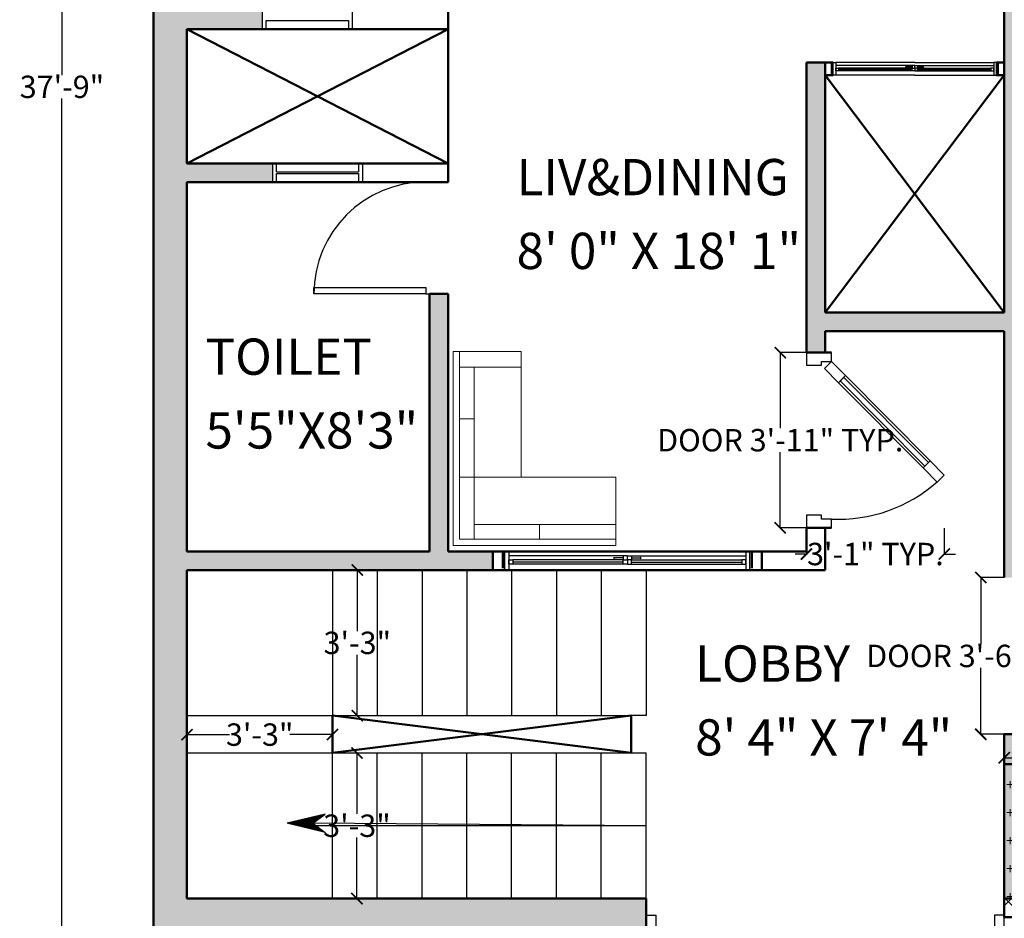
# Model space of a CAD drawing. Units: inches. Extents: x 2278 to 7495, y -71 to 1198.
# Tile 2 of 44: x 2278 to 2542, y 714 to 955. Entities that reach past the tile are written whole.
import ezdxf

# ---------------------------------------------------------------- set-up
doc = ezdxf.new("R2010")
doc.units = ezdxf.units.IN
doc.header["$MEASUREMENT"] = 0
for name, color, linetype, lineweight in [('A-ANNO-DIMS', 2, 'Continuous', 18), ('A-AREA-IDEN', 3, 'Continuous', 18), ('A-Door', 3, 'Continuous', 25), ('A-FLOR-PATT', 252, 'Continuous', 13), ('A-FLOR-STRS', 6, 'Continuous', 25), ('A-FURN', 8, 'Continuous', 18), ('A-Glaz', 4, 'Continuous', 25), ('A-Wall', 7, 'Continuous', 50), ('A-WALL-PATT', 8, 'Continuous', 18)]:
    doc.layers.add(name, color=color, linetype=linetype, lineweight=lineweight)
doc.styles.get("Standard").update_dxf_attribs({"font": 'arial.ttf'})
doc.dimstyles.get("Standard").update_dxf_attribs({"dimtxt": 6, "dimasz": 3, "dimexe": 0.18, "dimexo": 0.0625, "dimgap": 0.09, "dimtad": 0, "dimtih": 1, "dimtoh": 1, "dimdec": 0, "dimzin": 0, "dimdsep": 46, "dimlunit": 3, "dimtxsty": 'Standard', "dimblk": 'ARCHTICK', "dimcen": 0.09, "dimadec": 0, "dimazin": 0, "dimtfac": 1, "dimtdec": 0, "dimtofl": 0, "dimtmove": 0, "dimatfit": 3, "dimfxl": 1, "dimtolj": 1, "dimtzin": 0, "dimarcsym": 0})

# ---------------------------------------------------------------- blocks, each defined once
blk = doc.blocks.new('*U5')
for p, q in [((0, 0), (0, -6)), ((30, 0), (30, -6))]:
    blk.add_line(p, q)
blk.add_lwpolyline([(0, 0), (0, 30), (1.75, 30), (1.75, 0)], close=True)
blk.add_arc((0, 0), 30, 0, 90)
blk = doc.blocks.new('A$C58286AE3')
for p, q in [((75, 820), (35, 820)), ((35, 820), (35, 180)), ((65, 820), (45, 820)), ((75, 180), (75, 820)), ((75, 180), (35, 180)), ((35, 180), (75, 180)), ((45, 180), (65, 180))]:
    blk.add_line(p, q)
blk.add_lwpolyline([(1725, 180), (1725, 820), (1765, 820), (1765, 180)], close=True)
blk.add_arc((1756.5, 42.1), 858.5, 92.1038, 176.1334)
blk.add_ellipse((70, 105), major_axis=(-772.1, 325.5), ratio=0.94084, start_param=-2.726592, end_param=-1.199193)
at = {"layer": 'A-Door'}
for p, q in [((35, 820), (35, 900)), ((35, 900), (75, 900)), ((75, 900), (75, 820)), ((75, 820), (35, 820)), ((35, 180), (35, 100)), ((75, 100), (75, 180)), ((35, 100), (0, 100)), ((0, 100), (0, 0)), ((35, 60), (35, 100)), ((35, 100), (75, 100)), ((50, 60), (35, 60)), ((50, 50), (50, 60)), ((50, 0), (50, 50)), ((0, 0), (50, 0))]:
    blk.add_line(p, q, dxfattribs=at)
for points in [[(1725, 900), (1725, 820), (1765, 820), (1765, 900)], [(1725, 100), (1725, 180), (1765, 180), (1765, 100)], [(1765, 100), (1800, 100), (1800, 0), (1750, 0), (1750, 50), (1750, 60), (1765, 60)]]:
    blk.add_lwpolyline(points, close=True, dxfattribs=at)
at = {"layer": 'A-Glaz'}
for p, q in [((45, 820), (45, 180)), ((65, 180), (65, 820))]:
    blk.add_line(p, q, dxfattribs=at)
blk.add_lwpolyline([(1735, 180), (1735, 820), (1755, 820), (1755, 180)], close=True, dxfattribs=at)
blk = doc.blocks.new('A$C1DF4181C')
blk.add_lwpolyline([(120, 128), (460.7, 466.1), (432.5, 494.5), (91.8, 156.4)], close=True)
blk.add_arc((72.4, 128.7), 593.3, 357.2313, 41.4937)
at = {"layer": 'A-Door'}
for points in [[(517.5, 522.4), (460.7, 466.1), (432.5, 494.5), (489.3, 550.8)], [(63.2, 71.6), (120, 128), (91.8, 156.4), (35, 100)], [(35, 100), (0, 100), (0, 0), (50, 0), (50, 50), (50, 60), (35, 60)], [(665, 100), (665, 60), (650, 60), (650, 50), (650, 0), (700, 0), (700, 100)]]:
    blk.add_lwpolyline(points, close=True, dxfattribs=at)
at = {"layer": 'A-Glaz'}
blk.add_lwpolyline([(112.9, 135.1), (453.6, 473.2), (439.5, 487.4), (98.8, 149.3)], close=True, dxfattribs=at)
at = {"layer": 'A-Wall'}
for p, q in [((0, 0), (0, 100)), ((0, 100), (0, 0)), ((700, 0), (700, 100)), ((700, 0), (700, 100))]:
    blk.add_line(p, q, dxfattribs=at)
blk = doc.blocks.new('_ArchTick')
at = {"color": 0, "linetype": 'ByBlock', "const_width": 0.15}
blk.add_lwpolyline([(-0.5, -0.5), (0.5, 0.5)], dxfattribs=at)
blk = doc.blocks.new('*D11')
at = {"layer": 'A-ANNO-DIMS', "color": 0, "lineweight": -2, "transparency": 16777216}
for p, q in [((2367.65, 807.47), (2368.7, 807.47)), ((2368.52, 807.47), (2368.52, 791.12)), ((2368.52, 768.47), (2368.52, 784.81)), ((2367.65, 768.47), (2368.7, 768.47))]:
    blk.add_line(p, q, dxfattribs=at)
at = {"layer": 'Defpoints', "color": 0, "transparency": 16777216}
for p in [(2367.59, 807.47), (2367.59, 768.47), (2368.52, 768.47)]:
    blk.add_point(p, dxfattribs=at)
at = {"layer": 'A-ANNO-DIMS', "color": 0, "lineweight": -2, "transparency": 16777216, "xscale": 3, "yscale": 3, "zscale": 3}
for p, rotation in [((2368.52, 807.47), 90), ((2368.52, 768.47), 270)]:
    blk.add_blockref('_ArchTick', p, dxfattribs=dict(at, rotation=rotation))
at = {"layer": 'A-ANNO-DIMS', "color": 0, "transparency": 16777216, "insert": (2368.52, 787.97), "char_height": 6, "attachment_point": 5}
blk.add_mtext('\\A1;3\'-3"', dxfattribs=at)
blk = doc.blocks.new('*D12')
at = {"layer": 'A-ANNO-DIMS', "color": 0, "lineweight": -2, "transparency": 16777216}
for p, q in [((2322.87, 763.4), (2322.87, 763.21)), ((2322.87, 763.39), (2334.31, 763.39)), ((2361.87, 763.39), (2350.43, 763.39)), ((2361.87, 763.4), (2361.87, 763.21))]:
    blk.add_line(p, q, dxfattribs=at)
at = {"layer": 'Defpoints', "color": 0, "transparency": 16777216}
for p in [(2322.87, 763.47), (2361.87, 763.47), (2361.87, 763.39)]:
    blk.add_point(p, dxfattribs=at)
at = {"layer": 'A-ANNO-DIMS', "color": 0, "lineweight": -2, "transparency": 16777216, "xscale": 3, "yscale": 3, "zscale": 3, "rotation": 180}
blk.add_blockref('_ArchTick', (2322.87, 763.39), dxfattribs=at)
at = {"layer": 'A-ANNO-DIMS', "color": 0, "lineweight": -2, "transparency": 16777216, "xscale": 3, "yscale": 3, "zscale": 3}
blk.add_blockref('_ArchTick', (2361.87, 763.39), dxfattribs=at)
at = {"layer": 'A-ANNO-DIMS', "color": 0, "transparency": 16777216, "insert": (2342.37, 763.39), "char_height": 6, "attachment_point": 5}
blk.add_mtext('\\A1;3\'-3"', dxfattribs=at)
blk = doc.blocks.new('*D13')
at = {"layer": 'A-ANNO-DIMS', "color": 0, "lineweight": -2, "transparency": 16777216}
for p, q in [((2367.61, 758.47), (2368.61, 758.47)), ((2368.43, 758.47), (2368.43, 742.12)), ((2368.43, 719.47), (2368.43, 735.81)), ((2367.61, 719.47), (2368.61, 719.47))]:
    blk.add_line(p, q, dxfattribs=at)
at = {"layer": 'Defpoints', "color": 0, "transparency": 16777216}
for p in [(2367.55, 758.47), (2367.55, 719.47), (2368.43, 719.47)]:
    blk.add_point(p, dxfattribs=at)
at = {"layer": 'A-ANNO-DIMS', "color": 0, "lineweight": -2, "transparency": 16777216, "xscale": 3, "yscale": 3, "zscale": 3}
for p, rotation in [((2368.43, 758.47), 90), ((2368.43, 719.47), 270)]:
    blk.add_blockref('_ArchTick', p, dxfattribs=dict(at, rotation=rotation))
at = {"layer": 'A-ANNO-DIMS', "color": 0, "transparency": 16777216, "insert": (2368.43, 738.97), "char_height": 6, "attachment_point": 5}
blk.add_mtext('\\A1;3\'-3"', dxfattribs=at)
blk = doc.blocks.new('*D17')
at = {"layer": 'A-ANNO-DIMS', "color": 0, "lineweight": -2, "transparency": 16777216}
for p, q in [((2313.81, 1163.47), (2289.2, 1163.47)), ((2289.38, 1163.47), (2289.38, 940.12)), ((2289.38, 710.47), (2289.38, 933.81)), ((2313.81, 710.47), (2289.2, 710.47))]:
    blk.add_line(p, q, dxfattribs=at)
at = {"layer": 'Defpoints', "color": 0, "transparency": 16777216}
for p in [(2313.87, 1163.47), (2289.38, 710.47), (2313.87, 710.47)]:
    blk.add_point(p, dxfattribs=at)
at = {"layer": 'A-ANNO-DIMS', "color": 0, "lineweight": -2, "transparency": 16777216, "xscale": 3, "yscale": 3, "zscale": 3}
for p, rotation in [((2289.38, 1163.47), 90), ((2289.38, 710.47), 270)]:
    blk.add_blockref('_ArchTick', p, dxfattribs=dict(at, rotation=rotation))
at = {"layer": 'A-ANNO-DIMS', "color": 0, "transparency": 16777216, "insert": (2289.38, 936.97), "char_height": 6, "attachment_point": 5}
blk.add_mtext('\\A1;37\'-9"', dxfattribs=at)
blk = doc.blocks.new('*D43')
at = {"layer": 'A-ANNO-DIMS', "color": 0, "lineweight": -2, "transparency": 16777216}
for p, q in [((2541.81, 805.47), (2535.39, 805.47)), ((2535.57, 805.47), (2535.57, 787.66)), ((2535.57, 763.47), (2535.57, 781.27)), ((2541.81, 763.47), (2535.39, 763.47))]:
    blk.add_line(p, q, dxfattribs=at)
at = {"layer": 'Defpoints', "color": 0, "transparency": 16777216}
for p in [(2541.87, 805.47), (2535.57, 763.47), (2541.87, 763.47)]:
    blk.add_point(p, dxfattribs=at)
at = {"layer": 'A-ANNO-DIMS', "color": 0, "lineweight": -2, "transparency": 16777216, "xscale": 3, "yscale": 3, "zscale": 3}
for p, rotation in [((2535.57, 805.47), 90), ((2535.57, 763.47), 270)]:
    blk.add_blockref('_ArchTick', p, dxfattribs=dict(at, rotation=rotation))
at = {"layer": 'A-ANNO-DIMS', "color": 0, "transparency": 16777216, "insert": (2535.57, 784.47), "char_height": 6, "attachment_point": 5}
blk.add_mtext('\\A1;DOOR 3\'-6" TYP.', dxfattribs=at)
blk = doc.blocks.new('*D44')
at = {"layer": 'A-ANNO-DIMS', "color": 0, "lineweight": -2, "transparency": 16777216}
for p, q in [((2541.87, 763.4), (2541.87, 756.99)), ((2574.92, 763.4), (2574.92, 756.99)), ((2541.87, 757.17), (2574.92, 757.17)), ((2574.92, 757.17), (2577.92, 757.17))]:
    blk.add_line(p, q, dxfattribs=at)
at = {"layer": 'Defpoints', "color": 0, "transparency": 16777216}
for p in [(2541.87, 763.47), (2574.92, 763.47), (2574.92, 757.17)]:
    blk.add_point(p, dxfattribs=at)
at = {"layer": 'A-ANNO-DIMS', "color": 0, "lineweight": -2, "transparency": 16777216, "xscale": 3, "yscale": 3, "zscale": 3, "rotation": 180}
blk.add_blockref('_ArchTick', (2541.87, 757.17), dxfattribs=at)
at = {"layer": 'A-ANNO-DIMS', "color": 0, "lineweight": -2, "transparency": 16777216, "xscale": 3, "yscale": 3, "zscale": 3}
blk.add_blockref('_ArchTick', (2574.92, 757.17), dxfattribs=at)
at = {"layer": 'A-ANNO-DIMS', "color": 0, "transparency": 16777216, "insert": (2596.35, 757.17), "char_height": 6, "attachment_point": 5}
blk.add_mtext('\\A1;2\'-9" TYP.', dxfattribs=at)
blk = doc.blocks.new('*D47')
at = {"layer": 'A-ANNO-DIMS', "color": 0, "lineweight": -2, "transparency": 16777216}
for p, q in [((2488.81, 865.74), (2481.65, 865.74)), ((2481.83, 865.74), (2481.83, 845.48)), ((2481.83, 818.82), (2481.83, 839.08)), ((2488.81, 818.82), (2481.65, 818.82))]:
    blk.add_line(p, q, dxfattribs=at)
at = {"layer": 'Defpoints', "color": 0, "transparency": 16777216}
for p in [(2488.87, 865.74), (2481.83, 818.82), (2488.87, 818.82)]:
    blk.add_point(p, dxfattribs=at)
at = {"layer": 'A-ANNO-DIMS', "color": 0, "lineweight": -2, "transparency": 16777216, "xscale": 3, "yscale": 3, "zscale": 3}
for p, rotation in [((2481.83, 865.74), 90), ((2481.83, 818.82), 270)]:
    blk.add_blockref('_ArchTick', p, dxfattribs=dict(at, rotation=rotation))
at = {"layer": 'A-ANNO-DIMS', "color": 0, "transparency": 16777216, "insert": (2481.83, 842.28), "char_height": 6, "attachment_point": 5}
blk.add_mtext('\\A1;DOOR 3\'-11" TYP.', dxfattribs=at)
blk = doc.blocks.new('*D48')
at = {"layer": 'A-ANNO-DIMS', "color": 0, "lineweight": -2, "transparency": 16777216}
for p, q in [((2488.87, 818.75), (2488.87, 811.6)), ((2525.8, 818.75), (2525.8, 811.6)), ((2488.87, 811.78), (2485.87, 811.78)), ((2525.8, 811.78), (2528.8, 811.78))]:
    blk.add_line(p, q, dxfattribs=at)
at = {"layer": 'Defpoints', "color": 0, "transparency": 16777216}
for p in [(2488.87, 818.82), (2525.8, 818.82), (2525.8, 811.78)]:
    blk.add_point(p, dxfattribs=at)
at = {"layer": 'A-ANNO-DIMS', "color": 0, "lineweight": -2, "transparency": 16777216, "xscale": 3, "yscale": 3, "zscale": 3}
blk.add_blockref('_ArchTick', (2488.87, 811.78), dxfattribs=at)
at = {"layer": 'A-ANNO-DIMS', "color": 0, "lineweight": -2, "transparency": 16777216, "xscale": 3, "yscale": 3, "zscale": 3, "rotation": 180}
blk.add_blockref('_ArchTick', (2525.8, 811.78), dxfattribs=at)
at = {"layer": 'A-ANNO-DIMS', "color": 0, "transparency": 16777216, "insert": (2507.33, 811.78), "char_height": 6, "attachment_point": 5}
blk.add_mtext('\\A1;3\'-1" TYP.', dxfattribs=at)

msp = doc.modelspace()

# ---------------------------------------------------------------- hatches: boundary and pattern name
at = {"layer": 'A-FLOR-PATT'}
h = msp.add_hatch(dxfattribs=at)
h.set_pattern_fill('ANSI31', color=256)
h.paths.add_polyline_path([(2356.59, 739.64), (2359.92, 742.09), (2349.69, 739.64), (2359.92, 737.18)])
at = {"layer": 'A-WALL-PATT'}
h = msp.add_hatch(dxfattribs=at)
h.set_pattern_fill('ANSI36', color=256, scale=30)
h.paths.add_polyline_path([(2343.12, 957.47), (2322.87, 957.47), (2322.87, 1029.47), (2351.87, 1029.47), (2351.87, 1034.47), (2322.87, 1034.47), (2322.87, 1154.47), (2339.87, 1154.47), (2339.87, 1163.47), (2313.87, 1163.47), (2313.87, 710.47), (2445.87, 710.47), (2445.87, 719.47), (2322.87, 719.47), (2322.87, 807.47), (2404.87, 807.47), (2404.87, 812.47), (2392.87, 812.47), (2392.87, 881.47), (2387.87, 881.47), (2387.87, 812.47), (2322.87, 812.47), (2322.87, 911.47), (2345.87, 911.47), (2345.87, 916.47), (2322.87, 916.47), (2322.87, 952.47), (2343.12, 952.47)])
h.paths.add_polyline_path([(2451.87, 1163.47), (2411.87, 1163.47), (2411.87, 1154.47), (2428.87, 1154.47), (2428.87, 1034.47), (2428.87, 1029.47), (2433.87, 1029.47), (2433.87, 1154.47), (2451.87, 1154.47)])
h.paths.add_polyline_path([(2558.87, 1163.47), (2523.87, 1163.47), (2523.87, 1154.47), (2541.87, 1154.47), (2541.87, 1034.47), (2475.87, 1034.47), (2475.87, 1029.47), (2541.87, 1029.47), (2541.87, 943.47), (2541.87, 940.13), (2541.87, 876.47), (2493.87, 876.47), (2493.87, 943.47), (2488.87, 943.47), (2488.87, 871.47), (2488.87, 865.74), (2493.88, 865.74), (2493.88, 871.47), (2541.87, 871.47), (2541.87, 805.47), (2546.87, 805.47), (2546.87, 1077.47), (2558.87, 1077.47), (2558.87, 1082.47), (2546.87, 1082.47), (2546.87, 1154.47), (2558.87, 1154.47)])
h.paths.add_polyline_path([(2716.87, 937.97), (2707.87, 937.97), (2707.87, 911.47), (2594.87, 911.47), (2594.87, 906.47), (2707.87, 906.47), (2707.87, 869.47), (2716.87, 869.47)])
h.paths.add_polyline_path([(2716.87, 1163.47), (2689.87, 1163.47), (2689.87, 1154.47), (2707.87, 1154.47), (2707.87, 1041.47), (2594.87, 1041.47), (2594.87, 1036.47), (2707.87, 1036.47), (2707.87, 1009.97), (2716.87, 1009.97)])
h.paths.add_polyline_path([(2617.87, 1163.47), (2582.87, 1163.47), (2582.87, 1154.47), (2594.87, 1154.47), (2594.87, 1082.47), (2588.87, 1082.47), (2588.87, 1077.47), (2599.87, 1077.47), (2599.87, 1154.47), (2617.87, 1154.47)])
h.paths.add_polyline_path([(2716.87, 797.47), (2707.87, 797.47), (2707.87, 760.47), (2663.37, 760.47), (2663.37, 755.47), (2716.87, 755.47)])
h.paths.add_polyline_path([(2591.37, 760.47), (2546.87, 760.47), (2546.87, 763.47), (2541.87, 763.47), (2541.87, 755.47), (2591.37, 755.47)])
h = msp.add_hatch(dxfattribs=at)
h.set_pattern_fill('ANSI37', color=256, scale=30)
h.paths.add_polyline_path([(2716.87, 755.47), (2707.87, 755.47), (2707.87, 719.47), (2541.87, 719.47), (2541.87, 714.47), (2716.87, 714.47)])
at = {"layer": 'A-WALL-PATT', "transparency": 33554562}
h = msp.add_hatch(color=256, dxfattribs=at)
h.dxf.hatch_style = 1
h.paths.add_polyline_path([(2707.87, 755.47), (2541.87, 755.47), (2541.87, 719.47), (2707.87, 719.47)])
h = msp.add_hatch(dxfattribs=at)
h.set_pattern_fill('CROSS', color=256, scale=15)
h.paths.add_polyline_path([(2707.87, 755.47), (2541.87, 755.47), (2541.87, 719.47), (2707.87, 719.47)])

# ---------------------------------------------------------------- linework, layer by layer
at = {"layer": 'A-FLOR-STRS'}
for p, q in [((2361.87, 807.47), (2361.87, 768.47)), ((2373.87, 807.47), (2373.87, 768.47)), ((2385.87, 807.47), (2385.87, 768.47)), ((2397.87, 807.47), (2397.87, 768.47)), ((2409.87, 807.47), (2409.87, 768.47)), ((2421.87, 807.47), (2421.87, 768.47)), ((2433.87, 807.47), (2433.87, 768.47)), ((2445.87, 807.47), (2445.87, 768.47)), ((2322.87, 768.47), (2441.87, 768.47)), ((2445.87, 768.47), (2441.87, 768.47)), ((2322.87, 758.47), (2445.87, 758.47)), ((2361.87, 719.47), (2361.87, 758.47)), ((2373.87, 719.47), (2373.87, 758.47)), ((2385.87, 719.47), (2385.87, 758.47)), ((2397.87, 719.47), (2397.87, 758.47)), ((2409.87, 719.47), (2409.87, 758.47)), ((2421.87, 719.47), (2421.87, 758.47)), ((2433.87, 719.47), (2433.87, 758.47)), ((2445.87, 719.47), (2445.87, 758.47)), ((2359.92, 742.09), (2349.69, 739.64)), ((2356.59, 739.64), (2359.92, 742.09)), ((2359.92, 737.18), (2349.69, 739.64)), ((2445.87, 738.97), (2356.59, 739.64)), ((2356.59, 739.64), (2359.92, 737.18)), ((2445.87, 738.97), (2357.33, 738.97))]:
    msp.add_line(p, q, dxfattribs=at)
at = {"layer": 'A-FURN'}
for p, q in [((2394.21, 814.1), (2394.21, 866.04)), ((2412.45, 866.04), (2394.21, 866.04)), ((2395.9, 815.79), (2395.9, 866.04)), ((2412.45, 832.34), (2412.45, 866.04)), ((2412.45, 861.82), (2395.9, 861.82)), ((2399.79, 815.79), (2399.79, 861.82)), ((2399.79, 848.05), (2395.9, 848.05)), ((2437.83, 832.34), (2395.9, 832.34)), ((2437.83, 814.1), (2437.83, 832.34)), ((2399.79, 819.67), (2437.83, 819.67)), ((2417.35, 815.79), (2417.35, 819.67)), ((2395.9, 815.79), (2437.83, 815.79)), ((2437.83, 814.1), (2394.21, 814.1))]:
    msp.add_line(p, q, dxfattribs=at)
at = {"layer": 'A-Glaz'}
for p, q in [((2343.12, 952.47), (2343.12, 957.47)), ((2367.12, 957.47), (2367.12, 952.47)), ((2367.12, 952.47), (2343.12, 952.47)), ((2344.12, 952.47), (2344.12, 954.77)), ((2344.12, 954.77), (2366.12, 954.77)), ((2366.12, 954.77), (2366.12, 952.47)), ((2517.87, 943.47), (2496.72, 943.47)), ((2517.87, 942.66), (2496.72, 942.66)), ((2517.15, 941.94), (2497.44, 941.94)), ((2517.15, 942.3), (2515.59, 942.3)), ((2517.87, 943.47), (2539.02, 943.47)), ((2517.87, 942.66), (2539.02, 942.66)), ((2518.59, 942.3), (2520.15, 942.3)), ((2518.59, 941.94), (2538.3, 941.94)), ((2517.87, 940.13), (2496.72, 940.13)), ((2517.15, 941.58), (2497.44, 941.58)), ((2517.15, 941.22), (2497.44, 941.22)), ((2517.87, 940.13), (2539.02, 940.13)), ((2518.59, 941.58), (2538.3, 941.58)), ((2518.59, 941.22), (2538.3, 941.22)), ((2345.87, 916.47), (2369.87, 916.47)), ((2345.87, 911.47), (2345.87, 916.47)), ((2346.87, 914.17), (2346.87, 916.47)), ((2368.87, 916.47), (2368.87, 914.17)), ((2369.87, 916.47), (2369.87, 911.47)), ((2346.87, 914.17), (2368.87, 914.17)), ((2346.87, 911.47), (2346.87, 913.77)), ((2346.87, 913.77), (2368.87, 913.77)), ((2368.87, 913.77), (2368.87, 911.47)), ((2369.87, 911.47), (2345.87, 911.47)), ((2440.87, 812.47), (2409.15, 812.47)), ((2440.87, 811.26), (2409.15, 811.26)), ((2439.79, 810.18), (2410.23, 810.18)), ((2439.79, 810.72), (2437.46, 810.72)), ((2440.87, 812.47), (2472.59, 812.47)), ((2440.87, 811.26), (2472.59, 811.26)), ((2441.95, 810.72), (2444.28, 810.72)), ((2441.95, 810.18), (2471.51, 810.18)), ((2440.87, 807.47), (2409.15, 807.47)), ((2439.79, 809.64), (2410.23, 809.64)), ((2439.79, 809.09), (2410.23, 809.09)), ((2440.87, 807.47), (2472.59, 807.47)), ((2441.95, 809.64), (2471.51, 809.64)), ((2441.95, 809.09), (2471.51, 809.09))]:
    msp.add_line(p, q, dxfattribs=at)
for points in [[(2496.72, 940.13), (2496, 940.13), (2496, 943.47), (2496.72, 943.47)], [(2497.44, 941.22), (2496.72, 941.22), (2496.72, 941.94), (2497.44, 941.94)], [(2515.41, 942.3), (2515.59, 942.41), (2515.59, 942.19)], [(2517.15, 941.94), (2517.87, 941.94), (2517.87, 942.66), (2517.15, 942.66)], [(2517.87, 941.22), (2517.15, 941.22), (2517.15, 941.94), (2517.87, 941.94)], [(2518.59, 941.94), (2517.87, 941.94), (2517.87, 942.66), (2518.59, 942.66)], [(2517.87, 941.22), (2518.59, 941.22), (2518.59, 941.94), (2517.87, 941.94)], [(2520.33, 942.3), (2520.15, 942.41), (2520.15, 942.19)], [(2538.3, 941.22), (2539.02, 941.22), (2539.02, 941.94), (2538.3, 941.94)], [(2539.02, 940.13), (2539.74, 940.13), (2539.74, 943.47), (2539.02, 943.47)], [(2409.15, 807.47), (2408.06, 807.47), (2408.06, 812.47), (2409.15, 812.47)], [(2410.23, 809.09), (2409.15, 809.09), (2409.15, 810.18), (2410.23, 810.18)], [(2437.18, 810.72), (2437.46, 810.88), (2437.46, 810.56)], [(2439.79, 810.18), (2440.87, 810.18), (2440.87, 811.26), (2439.79, 811.26)], [(2440.87, 809.09), (2439.79, 809.09), (2439.79, 810.18), (2440.87, 810.18)], [(2441.95, 810.18), (2440.87, 810.18), (2440.87, 811.26), (2441.95, 811.26)], [(2440.87, 809.09), (2441.95, 809.09), (2441.95, 810.18), (2440.87, 810.18)], [(2444.56, 810.72), (2444.28, 810.88), (2444.28, 810.56)], [(2471.51, 809.09), (2472.59, 809.09), (2472.59, 810.18), (2471.51, 810.18)], [(2472.59, 807.47), (2473.68, 807.47), (2473.68, 812.47), (2472.59, 812.47)]]:
    msp.add_lwpolyline(points, close=True, dxfattribs=at)
at = {"layer": 'A-Wall'}
for p, q in [((2313.87, 1163.47), (2313.87, 710.47)), ((2392.87, 1029.47), (2392.87, 911.47)), ((2541.87, 1029.47), (2541.87, 943.47)), ((2322.87, 952.47), (2392.87, 952.47)), ((2322.87, 952.47), (2322.87, 916.47)), ((2392.87, 916.47), (2322.87, 952.47)), ((2322.87, 916.47), (2392.87, 952.47)), ((2488.87, 943.47), (2488.87, 871.47)), ((2493.87, 943.47), (2488.87, 943.47)), ((2493.87, 943.47), (2493.87, 876.47)), ((2493.87, 940.13), (2493.87, 943.47)), ((2496, 943.47), (2493.87, 943.47)), ((2495.64, 943.39), (2495.64, 940.49)), ((2539.74, 943.47), (2541.87, 943.47)), ((2540.1, 943.39), (2540.1, 940.49)), ((2541.87, 943.47), (2541.87, 876.47)), ((2541.87, 940.13), (2541.87, 943.47)), ((2496, 940.13), (2493.87, 940.13)), ((2493.87, 876.47), (2541.87, 940.13)), ((2541.87, 876.47), (2493.87, 940.13)), ((2539.74, 940.13), (2541.87, 940.13)), ((2322.87, 916.47), (2392.87, 916.47)), ((2322.87, 911.47), (2392.87, 911.47)), ((2322.87, 911.47), (2322.87, 812.47)), ((2387.87, 881.47), (2392.87, 881.47)), ((2387.87, 881.47), (2387.87, 812.47)), ((2392.87, 881.47), (2392.87, 812.47)), ((2493.87, 876.47), (2541.87, 876.47)), ((2488.87, 871.47), (2488.87, 865.74)), ((2493.87, 871.47), (2541.87, 871.47)), ((2493.88, 865.74), (2493.88, 871.47)), ((2541.87, 871.47), (2541.87, 805.47)), ((2488.87, 865.74), (2493.88, 865.74)), ((2488.87, 812.47), (2488.87, 818.82)), ((2488.87, 818.82), (2493.83, 818.82)), ((2493.83, 818.82), (2493.87, 812.47)), ((2322.87, 812.47), (2387.87, 812.47)), ((2392.87, 812.47), (2488.87, 812.47)), ((2404.87, 807.47), (2404.87, 812.47)), ((2408.06, 812.47), (2404.87, 812.47)), ((2407.52, 812.35), (2407.52, 808.01)), ((2473.68, 812.47), (2476.87, 812.47)), ((2474.22, 812.35), (2474.22, 808.01)), ((2476.87, 807.47), (2476.87, 812.47)), ((2493.87, 812.47), (2493.87, 807.47)), ((2322.87, 807.47), (2493.87, 807.47)), ((2322.87, 807.47), (2322.87, 719.47)), ((2408.06, 807.47), (2404.87, 807.47)), ((2473.68, 807.47), (2476.87, 807.47)), ((2361.87, 758.47), (2361.87, 768.47)), ((2361.87, 758.47), (2441.87, 768.47)), ((2441.87, 758.47), (2361.87, 768.47)), ((2441.87, 768.47), (2441.87, 758.47)), ((2546.87, 763.47), (2541.87, 763.47)), ((2541.87, 763.47), (2541.87, 755.47)), ((2541.87, 755.47), (2716.87, 755.47)), ((2541.87, 755.47), (2541.87, 719.47)), ((2322.87, 719.47), (2445.87, 719.47)), ((2445.87, 710.47), (2445.87, 719.47)), ((2541.87, 719.47), (2707.87, 719.47)), ((2541.87, 719.47), (2541.87, 714.47)), ((2541.87, 714.47), (2716.87, 714.47))]:
    msp.add_line(p, q, dxfattribs=at)

# ---------------------------------------------------------------- block references
at = {"layer": 'A-Door', "rotation": 89.99999999999999}
msp.add_blockref('*U5', (2386.87, 881.47), dxfattribs=at)
at = {"layer": 'A-Door'}
for name, p, xscale, yscale, zscale, rotation in [('A$C1DF4181C', (2488.87, 865.74), 0.0670393380383952, 0.0670393380383952, 0.0670393380383952, 270), ('A$C58286AE3', (2445.87, 714.97), -0.0533333333333331, 0.0533333333333331, 0.0533333333333331, 180)]:
    msp.add_blockref(name, p, dxfattribs=dict(at, xscale=xscale, yscale=yscale, zscale=zscale, rotation=rotation))

# ---------------------------------------------------------------- texts
at = {"layer": 'A-AREA-IDEN'}
for s, height, p in [('LIV&DINING', 9.72, (2411.19, 907.92)), ('8\' 0" X 18\' 1"', 9.7203, (2411.19, 888.15)), ('TOILET', 9.72, (2327.84, 859.81)), ('5\'5"X8\'3"', 9.72, (2327.84, 840.04)), ('LOBBY', 9.72, (2459.04, 777.56)), ('8\' 4" X 7\' 4"', 9.7203, (2459.04, 757.78))]:
    msp.add_text(s, height=height, dxfattribs=at).set_placement(p)

# ---------------------------------------------------------------- dimensions: what is measured, and where the dimension line sits
at = {"layer": 'A-ANNO-DIMS'}
for base, p1, p2, picture, middle in [((2289.38, 710.47), (2313.87, 1163.47), (2313.87, 710.47), '*D17', (2289.38, 936.97)), ((2368.52, 768.47), (2367.59, 807.47), (2367.59, 768.47), '*D11', (2368.52, 787.97)), ((2368.43, 719.47), (2367.55, 758.47), (2367.55, 719.47), '*D13', (2368.43, 738.97))]:
    dim = msp.add_linear_dim(base=base, p1=p1, p2=p2, angle=90, dimstyle='Standard', override={"dimclrd": 0, "dimclre": 0, "dimclrt": 0}, dxfattribs=at)
    dim.commit()
    dim.dimension.update_dxf_attribs({"geometry": picture, "text_midpoint": middle})
for base, p1, p2, picture, middle in [((2481.83, 818.82), (2488.87, 865.74), (2488.87, 818.82), '*D47', (2481.83, 842.28)), ((2535.57, 763.47), (2541.87, 805.47), (2541.87, 763.47), '*D43', (2535.57, 784.47))]:
    dim = msp.add_linear_dim(base=base, p1=p1, p2=p2, angle=270, text='DOOR <> TYP.', dimstyle='Standard', override={"dimdec": 1, "dimrnd": 0, "dimzin": 1, "dimlunit": 4, "dimfrac": 2}, dxfattribs=at)
    dim.commit()
    dim.dimension.update_dxf_attribs({"geometry": picture, "text_midpoint": middle})
for base, p1, p2, picture, middle in [((2525.8, 811.78), (2488.87, 818.82), (2525.8, 818.82), '*D48', (2507.33, 811.78)), ((2574.9182, 757.1665), (2541.87, 763.4665), (2574.9182, 763.4665), '*D44', (2596.3459, 757.1665))]:
    dim = msp.add_linear_dim(base=base, p1=p1, p2=p2, text='<> TYP.', dimstyle='Standard', override={"dimdec": 1, "dimrnd": 0, "dimzin": 1, "dimlunit": 4, "dimfrac": 2}, dxfattribs=at)
    dim.commit()
    dim.dimension.update_dxf_attribs({"geometry": picture, "text_midpoint": middle})
dim = msp.add_linear_dim(base=(2361.87, 763.39), p1=(2322.87, 763.47), p2=(2361.87, 763.47), dimstyle='Standard', override={"dimclrd": 0, "dimclre": 0, "dimclrt": 0}, dxfattribs=at)
dim.commit()
dim.dimension.update_dxf_attribs({"geometry": '*D12', "text_midpoint": (2342.37, 763.39)})

doc.saveas('drawing.dxf')
